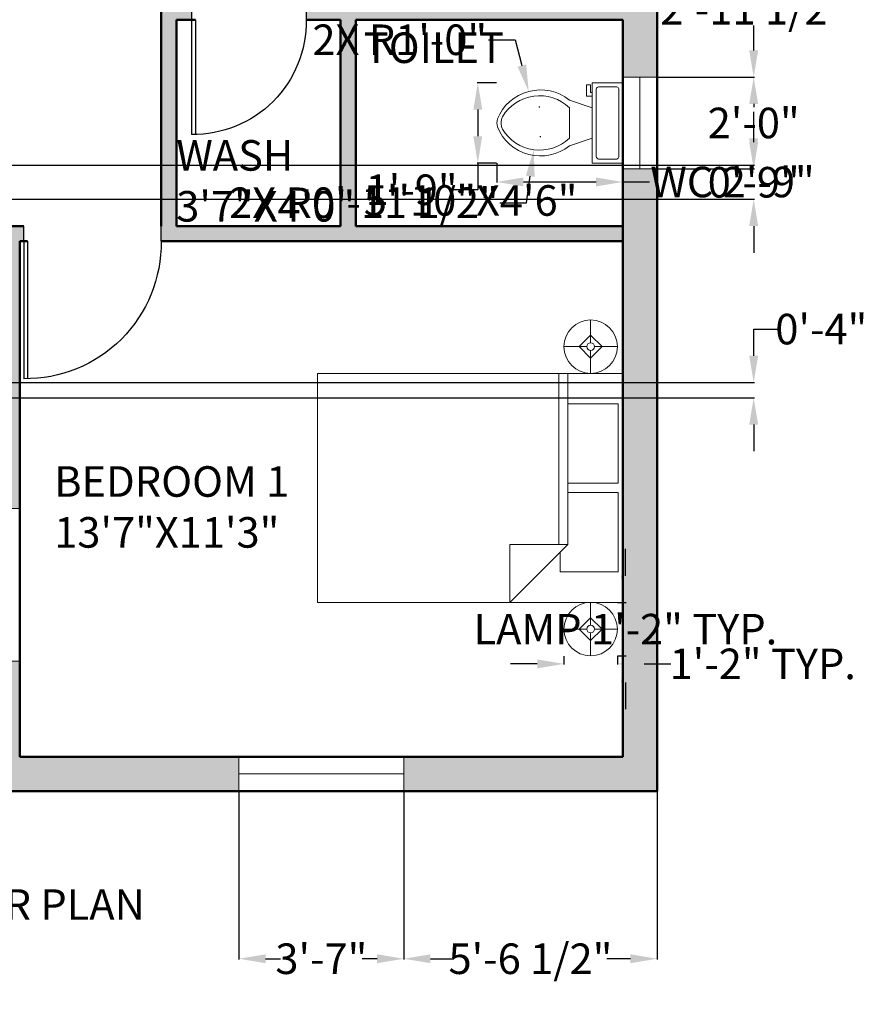
# Model space of a CAD drawing. Units: inches. Extents: x 808573 to 809030, y 884276 to 884799.
# Tile 2 of 4: x 808801 to 809023, y 884276 to 884534. Entities that reach past the tile are written whole.
import ezdxf

# ---------------------------------------------------------------- set-up
doc = ezdxf.new("R2010")
doc.units = ezdxf.units.IN
doc.header["$MEASUREMENT"] = 0
for name, color, linetype, lineweight in [('A-ANNO-DIMS', 2, 'Continuous', 18), ('A-ANNO-TEXT', 7, 'Continuous', 25), ('A-AREA-IDEN', 7, 'Continuous', 25), ('A-DOOR', 3, 'Continuous', 25), ('A-FLOR-FIXT', 9, 'Continuous', 18), ('A-FURN', 8, 'Continuous', 18), ('A-GLAZ', 4, 'Continuous', 18), ('A-WALL', 7, 'Continuous', 50)]:
    doc.layers.add(name, color=color, linetype=linetype, lineweight=lineweight)
doc.layers.add('A-WALL-PATT', color=251, linetype='Continuous', lineweight=13, true_color=0x636466)
doc.styles.get("Standard").update_dxf_attribs({"font": 'arial.ttf'})
doc.dimstyles.get("Standard").update_dxf_attribs({"dimtxt": 8, "dimasz": 7, "dimexe": 0.18, "dimexo": 0.0625, "dimgap": 0.09, "dimtad": 0, "dimtih": 1, "dimtoh": 1, "dimdec": 0, "dimzin": 0, "dimdsep": 46, "dimlunit": 3, "dimtxsty": 'Standard', "dimcen": 0.09, "dimadec": 0, "dimazin": 0, "dimtfac": 1, "dimtdec": 0, "dimtofl": 0, "dimtmove": 0, "dimatfit": 3, "dimfxl": 1, "dimtolj": 1, "dimtzin": 0, "dimarcsym": 0})

# ---------------------------------------------------------------- blocks, each defined once
blk = doc.blocks.new('Toilet - top')
for p, q in [((9.5, -6), (9.5, -2)), ((-10, -8.5), (-8, -8.5)), ((-10, -9.5), (-10, -8.5)), ((-7, -9.5), (-10, -9.5)), ((-8, -8.5), (-8, -8)), ((-7, -8), (-7, -9.5)), ((-4, -8), (-6, -14)), ((4, -8), (6, -14)), ((4, -14), (-4, -14))]:
    blk.add_line(p, q)
blk.add_lwpolyline([(10.5, -8), (10.5, 0), (-10.5, 0), (-10.5, -8)], close=True)
for points in [[(-9.5, -2), (-9.5, -6)], [(8.5, -1), (-8.5, -1)], [(-8.5, -7), (8.5, -7)]]:
    blk.add_lwpolyline(points)
for centre, radius, start, end in [((-8.62, -1.88), 0.884, 81.8699, 188.1301), ((8.62, -1.88), 0.884, 351.8699, 98.1301), ((-8.62, -6.12), 0.884, 171.8699, 278.1301), ((8.62, -6.12), 0.884, 261.8699, 8.1301), ((3.52, -21.58), 12.17, 141.4691, 247.9714), ((4.2, -21.82), 11.33, 136.3677, 238.9468), ((-3.52, -21.58), 12.17, 292.0284, 38.5307), ((-4.2, -21.82), 11.33, 301.053, 43.6321), ((0, -27.88), 4, 245.7318, 294.2682), ((0, -29), 4, 254.8605, 285.1395)]:
    blk.add_arc(centre, radius, start, end)
blk = doc.blocks.new('Bed - Queen')
for p, q in [((0, -80.00003), (0, 0)), ((0, 0), (59.99999, 0)), ((59.99999, 0), (59.99999, -80.00003)), ((7.99999, -1.2), (28.79998, -1.2)), ((7.99999, -14.4), (7.99999, -1.2)), ((28.79998, -1.2), (28.79998, -14.4)), ((31.19999, -1.2), (51.99999, -1.2)), ((31.19999, -14.4), (31.19999, -1.2)), ((51.99999, -1.2), (51.99999, -16.4)), ((0, -14.4), (44.8, -14.4)), ((59.99999, -29.6), (44.8, -14.4)), ((44.8, -14.4), (44.8, -29.6)), ((44.8, -16.8), (0, -16.8)), ((51.99999, -16.4), (46.79936, -16.4)), ((44.8, -29.6), (59.99999, -29.6)), ((59.99999, -80.00003), (0, -80.00003))]:
    blk.add_line(p, q)
blk = doc.blocks.new('Lamp - Table')
for p, q in [((0, 7), (0, 1)), ((0, 3), (-3, 0)), ((3, 0), (0, 3)), ((-1, 0), (-7, 0)), ((-3, 0), (0, -3)), ((0, -3), (3, 0)), ((1, 0), (7, 0)), ((0, -1), (0, -7))]:
    blk.add_line(p, q)
for radius in [7, 1]:
    blk.add_circle((0, 0), radius)
blk = doc.blocks.new('DOOR-SWING-36IN')
for p, q in [((0, 0), (0, 36)), ((1, 0), (1, 36)), ((0, 0), (0, -4)), ((36, 0), (36, -4))]:
    blk.add_line(p, q)
blk.add_arc((0.5, 0.5), 35.5, 359.1931, 90.8069)
blk = doc.blocks.new('DOOR-SWING-30IN')
for p, q in [((0, 30), (-4, 30)), ((-4, 1), (-34, 1)), ((-4, 0), (-34, 0)), ((0, 0), (-4, 0))]:
    blk.add_line(p, q)
blk.add_arc((-4.5, 0.5), 29.5, 89.029, 180.971)
blk = doc.blocks.new('WIN-40IN')
for p, q in [((0, 0), (9, 0)), ((4.5, 0), (4.5, -40)), ((0, -40), (9, -40))]:
    blk.add_line(p, q)
blk = doc.blocks.new('*D15')
at = {"layer": 'A-ANNO-DIMS', "color": 0, "lineweight": -2, "transparency": 16777216}
for p, q in [((808959.3, 884388.05), (808959.3, 884395.05)), ((808957.26, 884381.05), (808959.48, 884381.05)), ((808957.26, 884367.05), (808959.48, 884367.05)), ((808959.3, 884360.05), (808959.3, 884353.05))]:
    blk.add_line(p, q, dxfattribs=at)
at = {"layer": 'A-ANNO-DIMS', "color": 0, "transparency": 16777216}
for points in [[(808958.13, 884388.05), (808960.47, 884388.05), (808959.3, 884381.05)], [(808958.13, 884360.05), (808960.47, 884360.05), (808959.3, 884367.05)]]:
    blk.add_solid(points, dxfattribs=at)
at = {"layer": 'Defpoints', "color": 0, "transparency": 16777216}
for p in [(808957.2, 884381.05), (808959.3, 884381.05), (808957.2, 884367.05)]:
    blk.add_point(p, dxfattribs=at)
at = {"layer": 'A-ANNO-DIMS', "color": 0, "transparency": 16777216, "insert": (808959.3, 884374.05), "char_height": 8, "attachment_point": 5}
blk.add_mtext('\\A1;LAMP 1\'-2" TYP.', dxfattribs=at)
blk = doc.blocks.new('*D16')
at = {"layer": 'A-ANNO-DIMS', "color": 0, "lineweight": -2, "transparency": 16777216}
for p, q in [((808943.2, 884366.98), (808943.2, 884364.77)), ((808957.2, 884366.98), (808957.2, 884364.77)), ((808936.2, 884364.95), (808929.2, 884364.95)), ((808964.2, 884364.95), (808971.2, 884364.95))]:
    blk.add_line(p, q, dxfattribs=at)
at = {"layer": 'A-ANNO-DIMS', "color": 0, "transparency": 16777216}
for points in [[(808936.2, 884366.11), (808936.2, 884363.78), (808943.2, 884364.95)], [(808964.2, 884366.11), (808964.2, 884363.78), (808957.2, 884364.95)]]:
    blk.add_solid(points, dxfattribs=at)
at = {"layer": 'Defpoints', "color": 0, "transparency": 16777216}
for p in [(808943.2, 884367.05), (808957.2, 884367.05), (808957.2, 884364.95)]:
    blk.add_point(p, dxfattribs=at)
at = {"layer": 'A-ANNO-DIMS', "color": 0, "transparency": 16777216, "insert": (808995.3, 884364.95), "char_height": 8, "attachment_point": 5}
blk.add_mtext('\\A1;1\'-2" TYP.', dxfattribs=at)
blk = doc.blocks.new('*D27')
at = {"layer": 'A-ANNO-DIMS', "color": 0, "lineweight": -2, "transparency": 16777216}
for p, q in [((808925.58, 884496.08), (808925.58, 884491)), ((808958.63, 884496.08), (808958.63, 884491)), ((808932.58, 884491.18), (808951.63, 884491.18)), ((808958.63, 884491.18), (808965.63, 884491.18))]:
    blk.add_line(p, q, dxfattribs=at)
at = {"layer": 'A-ANNO-DIMS', "color": 0, "transparency": 16777216}
for points in [[(808932.58, 884492.35), (808932.58, 884490.02), (808925.58, 884491.18)], [(808951.63, 884492.35), (808951.63, 884490.02), (808958.63, 884491.18)]]:
    blk.add_solid(points, dxfattribs=at)
at = {"layer": 'Defpoints', "color": 0, "transparency": 16777216}
for p in [(808925.58, 884496.14), (808958.63, 884496.14), (808958.63, 884491.18)]:
    blk.add_point(p, dxfattribs=at)
at = {"layer": 'A-ANNO-DIMS', "color": 0, "transparency": 16777216, "insert": (808987.38, 884491.18), "char_height": 8, "attachment_point": 5}
blk.add_mtext('\\A1;WC 2\'-9"', dxfattribs=at)
blk = doc.blocks.new('*D28')
at = {"layer": 'A-ANNO-DIMS', "color": 0, "lineweight": -2, "transparency": 16777216}
for p, q in [((808925.52, 884517.14), (808920.45, 884517.14)), ((808920.63, 884510.14), (808920.63, 884503.14)), ((808925.52, 884496.14), (808920.45, 884496.14)), ((808920.63, 884496.14), (808920.63, 884489.14)), ((808920.63, 884489.14), (808913.63, 884489.14))]:
    blk.add_line(p, q, dxfattribs=at)
at = {"layer": 'A-ANNO-DIMS', "color": 0, "transparency": 16777216}
for points in [[(808919.46, 884510.14), (808921.79, 884510.14), (808920.63, 884517.14)], [(808919.46, 884503.14), (808921.79, 884503.14), (808920.63, 884496.14)]]:
    blk.add_solid(points, dxfattribs=at)
at = {"layer": 'Defpoints', "color": 0, "transparency": 16777216}
for p in [(808925.58, 884517.14), (808920.63, 884496.14), (808925.58, 884496.14)]:
    blk.add_point(p, dxfattribs=at)
at = {"layer": 'A-ANNO-DIMS', "color": 0, "transparency": 16777216, "insert": (808903.28, 884489.14), "char_height": 8, "attachment_point": 5}
blk.add_mtext('\\A1;1\'-9"', dxfattribs=at)
blk = doc.blocks.new('*D38')
at = {"layer": 'A-ANNO-DIMS', "color": 0, "lineweight": -2, "transparency": 16777216}
for p, q in [((808967.69, 884518.64), (808993.11, 884518.64)), ((808992.93, 884511.64), (808992.93, 884510.81)), ((808992.93, 884501.64), (808992.93, 884502.47)), ((808967.69, 884494.64), (808993.11, 884494.64))]:
    blk.add_line(p, q, dxfattribs=at)
at = {"layer": 'A-ANNO-DIMS', "color": 0, "transparency": 16777216}
for points in [[(808991.76, 884511.64), (808994.1, 884511.64), (808992.93, 884518.64)], [(808991.76, 884501.64), (808994.1, 884501.64), (808992.93, 884494.64)]]:
    blk.add_solid(points, dxfattribs=at)
at = {"layer": 'Defpoints', "color": 0, "transparency": 16777216}
for p in [(808967.63, 884518.64), (808992.93, 884518.64), (808967.63, 884494.64)]:
    blk.add_point(p, dxfattribs=at)
at = {"layer": 'A-ANNO-DIMS', "color": 0, "transparency": 16777216, "insert": (808992.93, 884506.64), "char_height": 8, "attachment_point": 5}
blk.add_mtext('\\A1;2\'-0"', dxfattribs=at)
blk = doc.blocks.new('*D39')
at = {"layer": 'A-ANNO-DIMS', "color": 0, "lineweight": -2, "transparency": 16777216}
for p, q in [((808967.69, 884554.14), (808993.11, 884554.14)), ((808992.93, 884547.14), (808992.93, 884540.62)), ((808992.93, 884525.64), (808992.93, 884532.16)), ((808967.69, 884518.64), (808993.11, 884518.64))]:
    blk.add_line(p, q, dxfattribs=at)
at = {"layer": 'A-ANNO-DIMS', "color": 0, "transparency": 16777216}
for points in [[(808991.76, 884547.14), (808994.1, 884547.14), (808992.93, 884554.14)], [(808991.76, 884525.64), (808994.1, 884525.64), (808992.93, 884518.64)]]:
    blk.add_solid(points, dxfattribs=at)
at = {"layer": 'Defpoints', "color": 0, "transparency": 16777216}
for p in [(808967.63, 884554.14), (808992.93, 884554.14), (808967.63, 884518.64)]:
    blk.add_point(p, dxfattribs=at)
at = {"layer": 'A-ANNO-DIMS', "color": 0, "transparency": 16777216, "insert": (808992.93, 884536.39), "char_height": 8, "attachment_point": 5}
blk.add_mtext('\\A1;2\'-11 1/2"', dxfattribs=at)
blk = doc.blocks.new('*D41')
at = {"layer": 'A-ANNO-DIMS', "color": 0, "lineweight": -2, "transparency": 16777216}
for p, q in [((808858.03, 884331.58), (808858.03, 884287.53)), ((808901.23, 884331.58), (808901.23, 884287.53)), ((808865.03, 884287.71), (808868.91, 884287.71)), ((808894.23, 884287.71), (808890.35, 884287.71))]:
    blk.add_line(p, q, dxfattribs=at)
at = {"layer": 'A-ANNO-DIMS', "color": 0, "transparency": 16777216}
for points in [[(808865.03, 884288.87), (808865.03, 884286.54), (808858.03, 884287.71)], [(808894.23, 884288.87), (808894.23, 884286.54), (808901.23, 884287.71)]]:
    blk.add_solid(points, dxfattribs=at)
at = {"layer": 'Defpoints', "color": 0, "transparency": 16777216}
for p in [(808858.03, 884331.64), (808901.23, 884331.64), (808901.23, 884287.71)]:
    blk.add_point(p, dxfattribs=at)
at = {"layer": 'A-ANNO-DIMS', "color": 0, "transparency": 16777216, "insert": (808879.63, 884287.71), "char_height": 8, "attachment_point": 5}
blk.add_mtext('\\A1;3\'-7"', dxfattribs=at)
blk = doc.blocks.new('*D42')
at = {"layer": 'A-ANNO-DIMS', "color": 0, "lineweight": -2, "transparency": 16777216}
for p, q in [((808901.23, 884331.58), (808901.23, 884287.53)), ((808967.63, 884331.58), (808967.63, 884287.53)), ((808908.23, 884287.71), (808914.38, 884287.71)), ((808960.63, 884287.71), (808954.47, 884287.71))]:
    blk.add_line(p, q, dxfattribs=at)
at = {"layer": 'A-ANNO-DIMS', "color": 0, "transparency": 16777216}
for points in [[(808908.23, 884288.87), (808908.23, 884286.54), (808901.23, 884287.71)], [(808960.63, 884288.87), (808960.63, 884286.54), (808967.63, 884287.71)]]:
    blk.add_solid(points, dxfattribs=at)
at = {"layer": 'Defpoints', "color": 0, "transparency": 16777216}
for p in [(808901.23, 884331.64), (808967.63, 884331.64), (808967.63, 884287.71)]:
    blk.add_point(p, dxfattribs=at)
at = {"layer": 'A-ANNO-DIMS', "color": 0, "transparency": 16777216, "insert": (808934.43, 884287.71), "char_height": 8, "attachment_point": 5}
blk.add_mtext('\\A1;5\'-6 1/2"', dxfattribs=at)
blk = doc.blocks.new('*D53')
at = {"layer": 'A-ANNO-DIMS', "color": 0, "lineweight": -2, "transparency": 16777216}
for p, q in [((808992.93, 884502.59), (808992.93, 884509.59)), ((808700.69, 884495.59), (808993.11, 884495.59)), ((808700.69, 884486.64), (808993.11, 884486.64)), ((808992.93, 884479.64), (808992.93, 884472.64))]:
    blk.add_line(p, q, dxfattribs=at)
at = {"layer": 'A-ANNO-DIMS', "color": 0, "transparency": 16777216}
for points in [[(808991.76, 884502.59), (808994.1, 884502.59), (808992.93, 884495.59)], [(808991.76, 884479.64), (808994.1, 884479.64), (808992.93, 884486.64)]]:
    blk.add_solid(points, dxfattribs=at)
at = {"layer": 'Defpoints', "color": 0, "transparency": 16777216}
for p in [(808700.63, 884495.59), (808992.93, 884495.59), (808700.63, 884486.64)]:
    blk.add_point(p, dxfattribs=at)
at = {"layer": 'A-ANNO-DIMS', "color": 0, "transparency": 16777216, "insert": (808992.93, 884491.11), "char_height": 8, "attachment_point": 5}
blk.add_mtext('\\A1;0\'-9"', dxfattribs=at)
blk = doc.blocks.new('*D54')
at = {"layer": 'A-ANNO-DIMS', "color": 0, "lineweight": -2, "transparency": 16777216}
for p, q in [((808992.93, 884445.64), (808992.93, 884452.64)), ((808992.93, 884452.64), (808999.93, 884452.64)), ((808704.69, 884438.64), (808993.11, 884438.64)), ((808704.69, 884434.64), (808993.11, 884434.64)), ((808992.93, 884427.64), (808992.93, 884420.64))]:
    blk.add_line(p, q, dxfattribs=at)
at = {"layer": 'A-ANNO-DIMS', "color": 0, "transparency": 16777216}
for points in [[(808991.76, 884445.64), (808994.1, 884445.64), (808992.93, 884438.64)], [(808991.76, 884427.64), (808994.1, 884427.64), (808992.93, 884434.64)]]:
    blk.add_solid(points, dxfattribs=at)
at = {"layer": 'Defpoints', "color": 0, "transparency": 16777216}
for p in [(808704.63, 884438.64), (808992.93, 884438.64), (808704.63, 884434.64)]:
    blk.add_point(p, dxfattribs=at)
at = {"layer": 'A-ANNO-DIMS', "color": 0, "transparency": 16777216, "insert": (809010.65, 884452.64), "char_height": 8, "attachment_point": 5}
blk.add_mtext('\\A1;0\'-4"', dxfattribs=at)
blk = doc.blocks.new('*D58')
at = {"layer": 'A-ANNO-DIMS', "color": 0, "lineweight": -2, "transparency": 16777216}
for p, q in [((808923.4, 884528.43), (808930.4, 884528.43)), ((808930.4, 884528.43), (808932.18, 884521.66)), ((808936.96, 884503.12), (808937.14, 884503.12)), ((808937.05, 884503.03), (808937.05, 884503.21))]:
    blk.add_line(p, q, dxfattribs=at)
at = {"layer": 'A-ANNO-DIMS', "color": 0, "transparency": 16777216}
blk.add_solid([(808933.31, 884521.96), (808931.05, 884521.36), (808933.96, 884514.89)], dxfattribs=at)
at = {"layer": 'Defpoints', "color": 0, "transparency": 16777216}
for p in [(808933.96, 884514.89), (808937.05, 884503.12)]:
    blk.add_point(p, dxfattribs=at)
at = {"layer": 'A-ANNO-DIMS', "color": 0, "transparency": 16777216, "insert": (808900.18, 884528.43), "char_height": 8, "attachment_point": 5}
blk.add_mtext('\\A1;2X R1\'-0"', dxfattribs=at)
blk = doc.blocks.new('*D59')
at = {"layer": 'A-ANNO-DIMS', "color": 0, "lineweight": -2, "transparency": 16777216}
for p, q in [((808936.72, 884510.84), (808936.9, 884510.84)), ((808936.81, 884510.75), (808936.81, 884510.93)), ((808933.43, 884485.74), (808934.37, 884492.67)), ((808926.43, 884485.74), (808933.43, 884485.74))]:
    blk.add_line(p, q, dxfattribs=at)
at = {"layer": 'A-ANNO-DIMS', "color": 0, "transparency": 16777216}
blk.add_solid([(808933.21, 884492.83), (808935.52, 884492.52), (808935.3, 884499.61)], dxfattribs=at)
at = {"layer": 'Defpoints', "color": 0, "transparency": 16777216}
for p in [(808936.81, 884510.84), (808935.3, 884499.61)]:
    blk.add_point(p, dxfattribs=at)
at = {"layer": 'A-ANNO-DIMS', "color": 0, "transparency": 16777216, "insert": (808890.79, 884485.74), "char_height": 8, "attachment_point": 5}
blk.add_mtext('\\A1;2X R0\'-11 1/2"', dxfattribs=at)

msp = doc.modelspace()

# ---------------------------------------------------------------- hatches: boundary and pattern name
at = {"layer": 'A-WALL-PATT'}
h = msp.add_hatch(color=256, dxfattribs=at)
h.dxf.hatch_style = 1
h.paths.add_polyline_path([(808967.63, 884751.64), (808619.63, 884751.64), (808619.63, 884696.64), (808628.63, 884696.64), (808628.63, 884742.64), (808791.63, 884742.64), (808958.63, 884742.64), (808958.63, 884696.64), (808967.63, 884696.64)])
h.paths.add_polyline_path([(808967.63, 884656.64), (808958.63, 884656.64), (808958.63, 884610.64), (808958.63, 884590.14), (808967.63, 884590.14)])
h.paths.add_polyline_path([(808967.63, 884494.64), (808958.63, 884494.64), (808958.63, 884479.64), (808958.63, 884340.64), (808901.23, 884340.64), (808901.23, 884331.64), (808967.63, 884331.64)])
h.paths.add_polyline_path([(808967.63, 884554.14), (808958.63, 884554.14), (808958.63, 884537.64), (808875.63, 884537.64), (808875.63, 884533.64), (808884.63, 884533.64), (808884.63, 884479.64), (808841.63, 884479.64), (808841.63, 884533.64), (808845.63, 884533.64), (808845.63, 884537.64), (808837.63, 884537.64), (808837.63, 884479.64), (808837.63, 884475.64), (808958.63, 884475.64), (808958.63, 884479.64), (808888.63, 884479.64), (808888.63, 884533.64), (808958.63, 884533.64), (808958.63, 884518.64), (808967.63, 884518.64)])
h.paths.add_polyline_path([(808858.03, 884340.64), (808800.63, 884340.64), (808800.63, 884365.64), (808791.63, 884365.64), (808791.63, 884331.64), (808858.03, 884331.64)])
h.paths.add_polyline_path([(808800.63, 884475.64), (808801.63, 884475.64), (808801.63, 884479.64), (808791.63, 884479.64), (808791.63, 884430.64), (808791.63, 884405.64), (808800.63, 884405.64)])
h.paths.add_polyline_path([(808740.63, 884434.64), (808704.63, 884434.64), (808704.63, 884438.64), (808700.63, 884438.64), (808700.63, 884434.64), (808628.63, 884434.64), (808628.63, 884443.64), (808619.63, 884443.64), (808619.63, 884430.64), (808740.63, 884430.64)])
h.paths.add_polyline_path([(808628.63, 884528.64), (808619.63, 884528.64), (808619.63, 884473.64), (808628.63, 884473.64), (808628.63, 884482.64)])
h.paths.add_polyline_path([(808628.63, 884606.64), (808628.63, 884656.64), (808619.63, 884656.64), (808619.63, 884564.64), (808628.63, 884564.64)])
h.paths.add_polyline_path([(808704.63, 884482.64), (808704.63, 884495.59), (808700.63, 884495.59), (808700.63, 884486.64), (808628.63, 884486.64), (808628.63, 884482.64), (808700.63, 884482.64), (808700.63, 884468.64), (808704.63, 884468.64)])
h.paths.add_polyline_path([(808704.63, 884606.64), (808700.63, 884606.64), (808700.63, 884531.59), (808704.63, 884531.59)])
h.paths.add_polyline_path([(808746.63, 884610.64), (808628.63, 884610.64), (808628.63, 884606.64), (808746.63, 884606.64)])
h.paths.add_polyline_path([(808804.63, 884610.64), (808795.63, 884610.64), (808795.63, 884742.64), (808791.63, 884742.64), (808791.63, 884610.64), (808782.63, 884610.64), (808782.63, 884606.64), (808804.63, 884606.64)])
h.paths.add_polyline_path([(808958.63, 884610.64), (808840.63, 884610.64), (808840.63, 884606.64), (808958.63, 884606.64)])

# ---------------------------------------------------------------- linework, layer by layer
at = {"layer": 'A-GLAZ'}
for p, q in [((808958.63, 884518.64), (808967.63, 884518.64)), ((808963.13, 884518.64), (808963.13, 884494.64)), ((808958.63, 884494.64), (808967.63, 884494.64)), ((808858.03, 884340.64), (808858.03, 884331.64)), ((808901.23, 884340.64), (808901.23, 884331.64)), ((808858.03, 884336.14), (808901.23, 884336.14))]:
    msp.add_line(p, q, dxfattribs=at)
at = {"layer": 'A-WALL'}
for p, q in [((808967.63, 884751.64), (808967.63, 884331.64)), ((808837.63, 884537.64), (808837.63, 884479.64)), ((808841.63, 884533.64), (808841.63, 884479.64)), ((808846.63, 884533.64), (808841.63, 884533.64)), ((808884.63, 884533.64), (808875.63, 884533.64)), ((808884.63, 884533.64), (808884.63, 884479.64)), ((808958.63, 884533.64), (808888.63, 884533.64)), ((808888.63, 884533.64), (808888.63, 884479.64)), ((808958.63, 884533.64), (808958.63, 884479.64)), ((808801.63, 884479.64), (808791.63, 884479.64)), ((808884.63, 884479.64), (808841.63, 884479.64)), ((808958.63, 884479.64), (808888.63, 884479.64)), ((808958.63, 884479.64), (808958.63, 884340.64)), ((808800.63, 884340.64), (808800.63, 884475.64)), ((808802.63, 884475.64), (808800.63, 884475.64)), ((808958.63, 884475.64), (808837.63, 884475.64)), ((808958.63, 884340.64), (808800.63, 884340.64)), ((808958.63, 884340.64), (808800.63, 884340.64)), ((808967.63, 884331.64), (808619.63, 884331.64))]:
    msp.add_line(p, q, dxfattribs=at)

# ---------------------------------------------------------------- block references
at = {"layer": 'A-DOOR', "extrusion": (0, 0, -1), "zscale": -1}
for name, p, rotation in [('DOOR-SWING-30IN', (-808845.63, 884537.64), 89.99999999926234), ('DOOR-SWING-36IN', (-808801.63, 884475.64), 180)]:
    msp.add_blockref(name, p, dxfattribs=dict(at, rotation=rotation))
at = {"layer": 'A-FLOR-FIXT', "rotation": 270}
msp.add_blockref('Toilet - top', (808958.63, 884506.64), dxfattribs=at)
at = {"layer": 'A-FURN', "rotation": 270}
for name, p in [('Lamp - Table', (808950.2, 884448.05)), ('Bed - Queen', (808958.63, 884441.05))]:
    msp.add_blockref(name, p, dxfattribs=at)
at = {"layer": 'A-FURN', "xscale": -1, "rotation": 270}
msp.add_blockref('Lamp - Table', (808950.2, 884374.05), dxfattribs=at)
at = {"layer": 'A-GLAZ'}
msp.add_blockref('WIN-40IN', (808791.63, 884405.64), dxfattribs=at)

# ---------------------------------------------------------------- texts
at = {"layer": 'A-ANNO-TEXT', "insert": (808720.2, 884305.91), "char_height": 8, "attachment_point": 1}
msp.add_mtext_dynamic_manual_height_columns('{\\fArial|b1|i0|c0|p34;GROUND FLOOR PLAN}', width=273.1721, gutter_width=1, heights=[0], dxfattribs=at)
at = {"layer": 'A-AREA-IDEN', "char_height": 8, "attachment_point": 1}
for s, insert in [('TOILET\\P\\P\\P5\'\'10"X4\'6"', (808890.75, 884530.34)), ('WASH\\P3\'7"X4\'0"', (808841.6, 884502.14)), ('BEDROOM 1\\P13\'7"X11\'3"', (808809.62, 884416.72))]:
    msp.add_mtext_dynamic_manual_height_columns(s, width=94.1107, gutter_width=1, heights=[0], dxfattribs=dict(at, insert=insert))

# ---------------------------------------------------------------- dimensions: what is measured, and where the dimension line sits
at = {"layer": 'A-ANNO-DIMS'}
for base, p1, p2, angle, picture, middle in [((808992.93, 884554.14), (808967.63, 884518.64), (808967.63, 884554.14), 90, '*D39', (808992.93, 884536.39)), ((808992.93, 884518.64), (808967.63, 884494.64), (808967.63, 884518.64), 90, '*D38', (808992.93, 884506.64)), ((808920.63, 884496.14), (808925.58, 884517.14), (808925.58, 884496.14), 270, '*D28', (808903.28, 884489.14)), ((808992.9284, 884495.5872), (808700.6284, 884486.64), (808700.6284, 884495.5872), 90, '*D53', (808992.9284, 884491.1136)), ((808992.93, 884438.64), (808704.63, 884434.64), (808704.63, 884438.64), 90, '*D54', (809010.65, 884452.64))]:
    dim = msp.add_linear_dim(base=base, p1=p1, p2=p2, angle=angle, dimstyle='Standard', override={"dimdec": 1, "dimlfac": 1, "dimrnd": 0, "dimzin": 1, "dimdsep": 46, "dimlunit": 4, "dimfrac": 2}, dxfattribs=at)
    dim.commit()
    dim.dimension.update_dxf_attribs({"geometry": picture, "text_midpoint": middle})
for center, mpoint, picture, middle in [((808937.05, 884503.12), (808933.96, 884514.89), '*D58', (808900.18, 884528.43)), ((808936.81, 884510.84), (808935.3, 884499.61), '*D59', (808890.79, 884485.74))]:
    dim = msp.add_radius_dim(center=center, mpoint=mpoint, text='2X <>', dimstyle='Standard', override={"dimdec": 1, "dimlfac": 1, "dimrnd": 0, "dimzin": 1, "dimdsep": 46, "dimlunit": 4, "dimfrac": 2}, dxfattribs=at)
    dim.commit()
    dim.dimension.update_dxf_attribs({"geometry": picture, "text_midpoint": middle})
for base, p1, p2, text, picture, middle in [((808958.6284, 884491.183), (808925.5822, 884496.14), (808958.6284, 884496.14), 'WC <>', '*D27', (808987.3773, 884491.183)), ((808957.2, 884364.95), (808943.2, 884367.05), (808957.2, 884367.05), '<> TYP.', '*D16', (808995.3, 884364.95))]:
    dim = msp.add_linear_dim(base=base, p1=p1, p2=p2, text=text, dimstyle='Standard', override={"dimdec": 1, "dimlfac": 1, "dimrnd": 0, "dimzin": 1, "dimdsep": 46, "dimlunit": 4, "dimfrac": 2}, dxfattribs=at)
    dim.commit()
    dim.dimension.update_dxf_attribs({"geometry": picture, "text_midpoint": middle})
dim = msp.add_linear_dim(base=(808959.3, 884381.05), p1=(808957.2, 884367.05), p2=(808957.2, 884381.05), angle=90, text='LAMP <> TYP.', dimstyle='Standard', override={"dimdec": 1, "dimlfac": 1, "dimrnd": 0, "dimzin": 1, "dimdsep": 46, "dimlunit": 4, "dimfrac": 2}, dxfattribs=at)
dim.commit()
dim.dimension.update_dxf_attribs({"geometry": '*D15', "text_midpoint": (808959.3, 884374.05)})
for base, p1, p2, picture, middle in [((808901.23, 884287.71), (808858.03, 884331.64), (808901.23, 884331.64), '*D41', (808879.63, 884287.71)), ((808967.63, 884287.71), (808901.23, 884331.64), (808967.63, 884331.64), '*D42', (808934.43, 884287.71))]:
    dim = msp.add_linear_dim(base=base, p1=p1, p2=p2, dimstyle='Standard', override={"dimdec": 1, "dimlfac": 1, "dimrnd": 0, "dimzin": 1, "dimdsep": 46, "dimlunit": 4, "dimfrac": 2}, dxfattribs=at)
    dim.commit()
    dim.dimension.update_dxf_attribs({"geometry": picture, "text_midpoint": middle})

doc.saveas('drawing.dxf')
